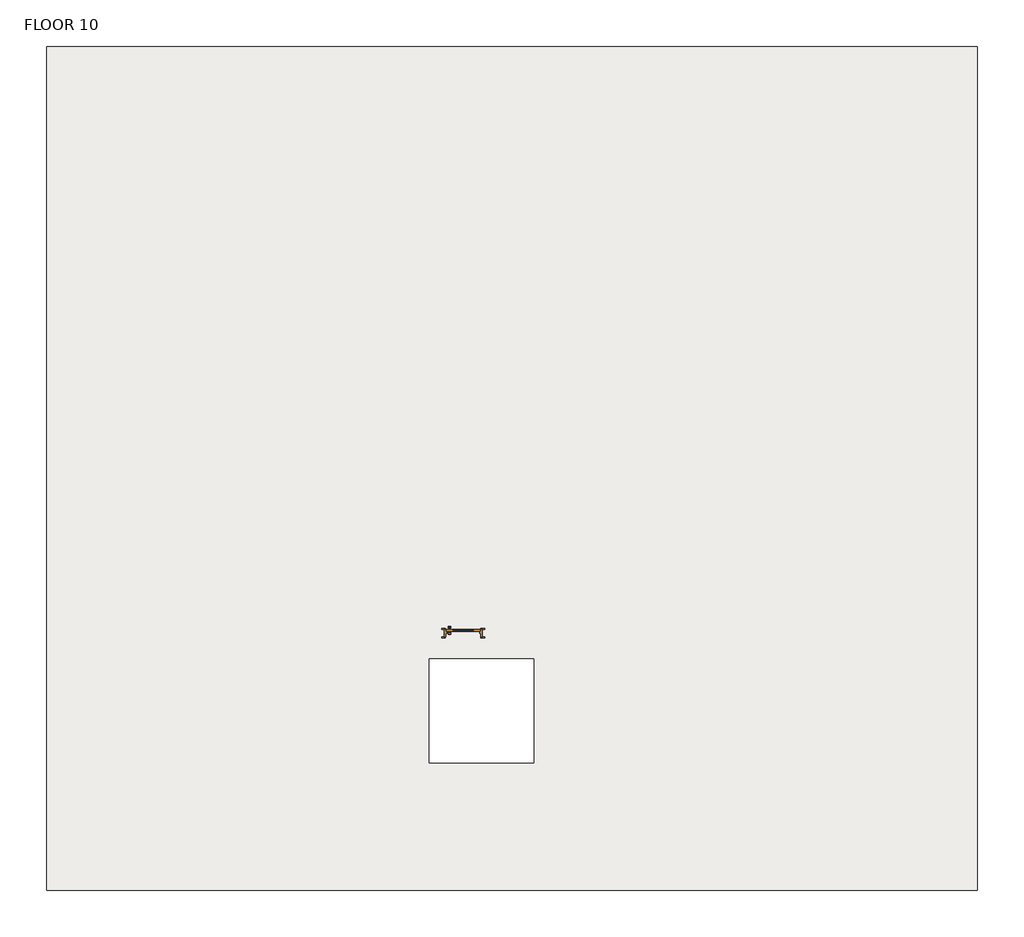
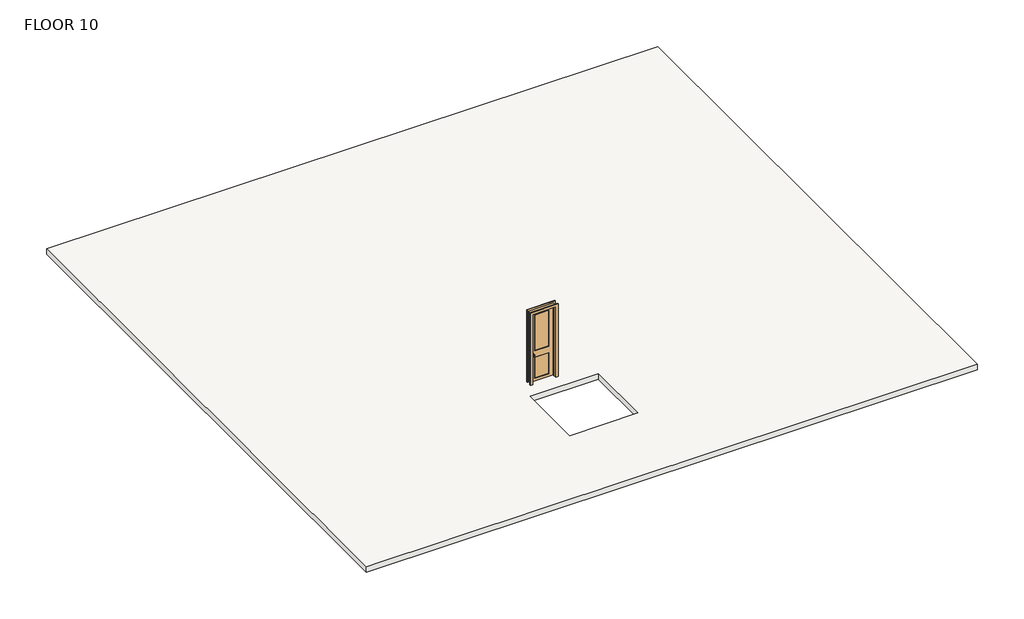
# One storey: 1 door, 1 roof.
"""IFC4 building model written with IfcOpenShell, lengths in millimetres."""

from ifc_helpers import new_model, si_unit, frame, origin, place, context, project, spatial, polyline, outline, extrude, transform, mapped, element, save
from components import door_596d7c92

model = new_model("IFC4")

# Units and contexts
model_context = context("Model", 3, world=origin())
ifc_project = project(units=[si_unit("LENGTHUNIT", "METRE", prefix="MILLI")], contexts=[model_context])

# Site, building, storey
site = spatial("IfcSite", under=ifc_project)
building = spatial("IfcBuilding", under=site)
storey = spatial("IfcBuildingStorey", under=building, Name="FLOOR 10", Elevation=15792.7725604)

# Door
placement = place(None, origin())
door_shape = door_596d7c92(model_context)
element("IfcDoor", 1, ObjectType="Door-Interior-Single-2_Panel-Wood : 24\" x 84\"", at=placement, inside=storey, context=model_context, shape_type="MappedRepresentation", body=[
    mapped(door_shape, transform((-5119.9094527, -3306.8492565, 15792.7725604), x_axis=(1.0, 0.0, 0.0), y_axis=(0.0, 1.0, 0.0), z_axis=(0.0, 0.0, 1.0))),
])

# Roof
element("IfcRoof", 2, ObjectType="ROOFING 6\"", at=placement, inside=storey, context=model_context, shape_type="SweptSolid", body=[
    extrude(outline(polyline([(3901.7862669, 6987.3281164), (3901.7862669, -7822.4593836), (-12430.4137331, -7822.4593836), (-12430.4137331, 6987.3281164), (3901.7862669, 6987.3281164)]), holes=[polyline([(-3883.9282812, -3760.9995759), (-5712.7282812, -3760.9995759), (-5712.7282812, -5589.7995759), (-3883.9282812, -5589.7995759), (-3883.9282812, -3760.9995759)])]), frame((0.0, 0.0, 15792.7725604), z_axis=(0.0, 0.0, 1.0), x_axis=(1.0, 0.0, 0.0)), (0.0, 0.0, 1.0), 152.4),
])

save(model, "model.ifc")

# Revit data of these elements
# Type "Door-Interior-Single-2_Panel-Wood : 24\" x 84\""
#   Type Mark = "10"
#   Assembly Code = "C1020300"
#   Analytic Construction = "Wooden"
#   Top Rail = 0' - 4 11/16"
#   Thickness = 0' - 1 3/8"
#   Thermal Resistance (R) = 2.5876 (h·ft²·°F)/BTU
#   Swing Angle [instance default] = 90.00°
#   Stiles = 0' - 4 3/4"
#   Rough Width = 2' - 2"
#   Rough Height = 7' - 1"
#   Lock Rail = 0' - 7 1/2"
#   Height = 7' - 0"
#   Width = 2' - 0"
#   Heat Transfer Coefficient (U) = 0.3865 BTU/(h·ft²·°F)
#   Bottom Rail = 0' - 9 1/8"
#   Trim Material = Cherry
#   Panel Material = Cherry
#   Frame Material = Cherry
#   Door Handle Material = Aluminum
#   Visual Light Transmittance = 0
#   Solar Heat Gain Coefficient = 0
#   Wall Closure = (empty or 0)
#   Function = (empty or 0)
# Type "ROOFING 6\""
#   Assembly Code = "B1020"
#   Layers, outside or top first: 0' - 6" no material (function 1)
# Element 1 (IfcDoor, "Door-Interior-Single-2_Panel-Wood : 24\" x 84\"")
#   Swing Angle = 90.00°
#   Phase Created = New Construction
#   Materials on its faces: "Cherry", "Aluminum"
# Element 2 (IfcRoof, "ROOFING 6\"")
#   built-in parameter 1001705 = 52.3136 (stored number, unit not read)
#   built-in parameter 1001710 = 33615
#   Phase Created = New Construction
#   Materials on its faces: "Default Roof"
# Materials
#   "Cherry": class "Wood", colour RGB 226 177 128, transparency 0, Description = "Prunus Serotina", Cost = 0
#   "Aluminum": class "Metal", colour RGB 247 247 247, transparency 0, Description = "Aluminum 6061", Cost = 0
#   "Default Roof": colour RGB 88 101 114, transparency 0, Cost = 0
